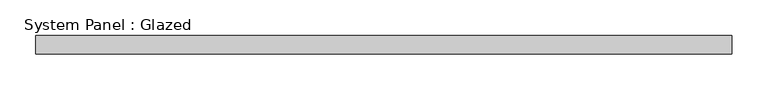
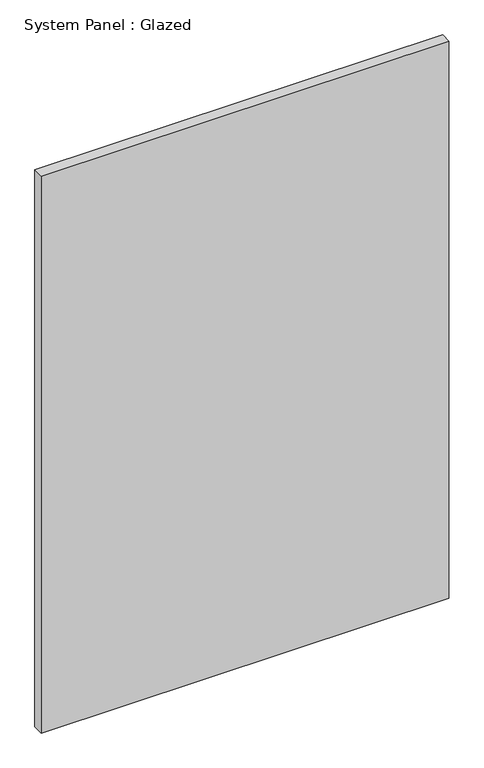
"""IFC4 building model written with IfcOpenShell, lengths in millimetres: plate geometry, System Panel : Glazed."""

from ifc_helpers import new_model, si_unit, origin, origin_with_axes, place, context, project, spatial, polyline, outline, extrude, source, transform, mapped, element, save


def system_panel_glazed_5228c6df(model_context):
    return source(origin(), model_context, "Body", "SweptSolid", [
        extrude(outline(polyline([(485.775, 19.05), (-485.775, 19.05), (-485.775, 44.45), (485.775, 44.45), (485.775, 19.05)])), origin_with_axes(), (0.0, 0.0, 1.0), 1402.8884341),
    ])


if __name__ == "__main__":
    model = new_model("IFC4")
    model_context = context("Model", 3, world=origin())
    ifc_project = project(units=[si_unit("LENGTHUNIT", "METRE", prefix="MILLI")], contexts=[model_context])
    site = spatial("IfcSite", under=ifc_project)
    building = spatial("IfcBuilding", under=site)
    placement = place(None, origin())
    system_panel_glazed_shape = system_panel_glazed_5228c6df(model_context)
    element("IfcPlate", 1, ObjectType="System Panel : Glazed", at=placement, inside=building, context=model_context, shape_type="MappedRepresentation", body=[
        mapped(system_panel_glazed_shape, transform((0.0, 0.0, 0.0), x_axis=(1.0, 0.0, 0.0), y_axis=(0.0, 1.0, 0.0), z_axis=(0.0, 0.0, 1.0))),
    ])
    save(model, "model.ifc")

# Revit data of these elements
# Type "System Panel : Glazed"
#   Construction Type Id = "GSP4R"
#   Analytic Construction = "1/8 in Pilkington single glazing"
#   Visual Light Transmittance = 0.9
#   Solar Heat Gain Coefficient = 0.86
#   Heat Transfer Coefficient (U) = 1.18115 BTU/(h·ft²·°F)
#   Define Thermal Properties by = 1
# Element 1 (IfcPlate, "System Panel : Glazed")
#   Materials on its faces: "Glass"
# Materials
#   "Glass": class "Glass", colour RGB 0 128 192, transparency 0.75, Description = "Soda Lime Glass", Cost = 0
